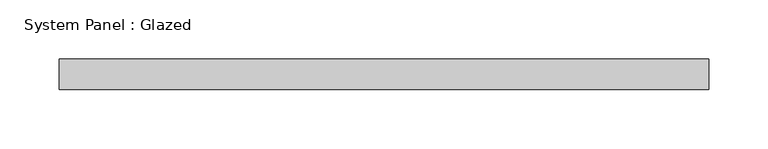
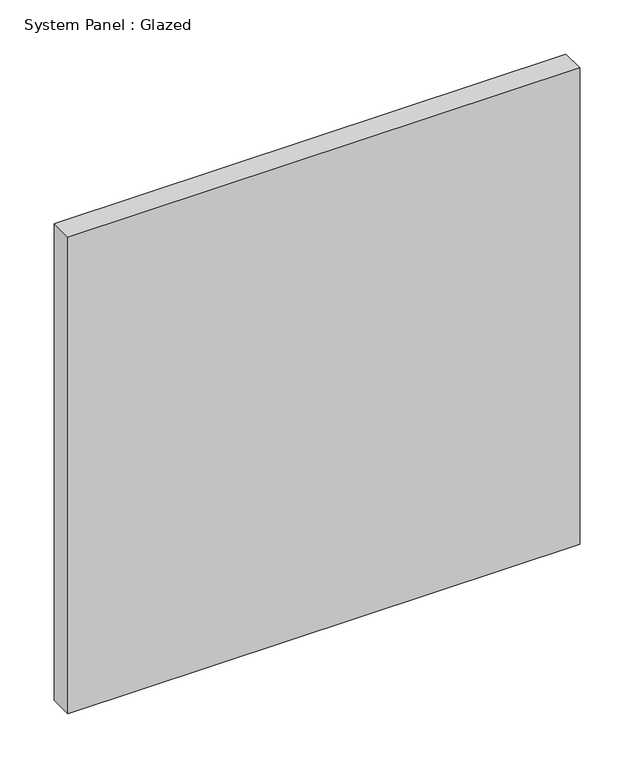
"""IFC4 building model written with IfcOpenShell, lengths in millimetres: plate geometry, System Panel : Glazed."""

from ifc_helpers import new_model, si_unit, origin, origin_with_axes, place, context, project, spatial, polyline, outline, extrude, source, transform, mapped, element, save


def system_panel_glazed_ec18a58b(model_context):
    return source(origin(), model_context, "Body", "SweptSolid", [
        extrude(outline(polyline([(273.05, 19.05), (-273.05, 19.05), (-273.05, 44.45), (273.05, 44.45), (273.05, 19.05)])), origin_with_axes(), (0.0, 0.0, 1.0), 537.6333333),
    ])


if __name__ == "__main__":
    model = new_model("IFC4")
    model_context = context("Model", 3, world=origin())
    ifc_project = project(units=[si_unit("LENGTHUNIT", "METRE", prefix="MILLI")], contexts=[model_context])
    site = spatial("IfcSite", under=ifc_project)
    building = spatial("IfcBuilding", under=site)
    placement = place(None, origin())
    system_panel_glazed_shape = system_panel_glazed_ec18a58b(model_context)
    element("IfcPlate", 1, ObjectType="System Panel : Glazed", at=placement, inside=building, context=model_context, shape_type="MappedRepresentation", body=[
        mapped(system_panel_glazed_shape, transform((0.0, 0.0, 0.0), x_axis=(1.0, 0.0, 0.0), y_axis=(0.0, 1.0, 0.0), z_axis=(0.0, 0.0, 1.0))),
    ])
    save(model, "model.ifc")

# Revit data of these elements
# Type "System Panel : Glazed"
#   Construction Type Id = "GSP4R"
#   Analytic Construction = "1/8 in Pilkington single glazing"
#   Visual Light Transmittance = 0.9
#   Solar Heat Gain Coefficient = 0.86
#   Heat Transfer Coefficient (U) = 1.18115 BTU/(h·ft²·°F)
#   Define Thermal Properties by = 1
# Element 1 (IfcPlate, "System Panel : Glazed")
#   Materials on its faces: "Glass"
# Materials
#   "Glass": class "Glass", colour RGB 0 128 192, transparency 0.75, Description = "Soda Lime Glass", Cost = 0
